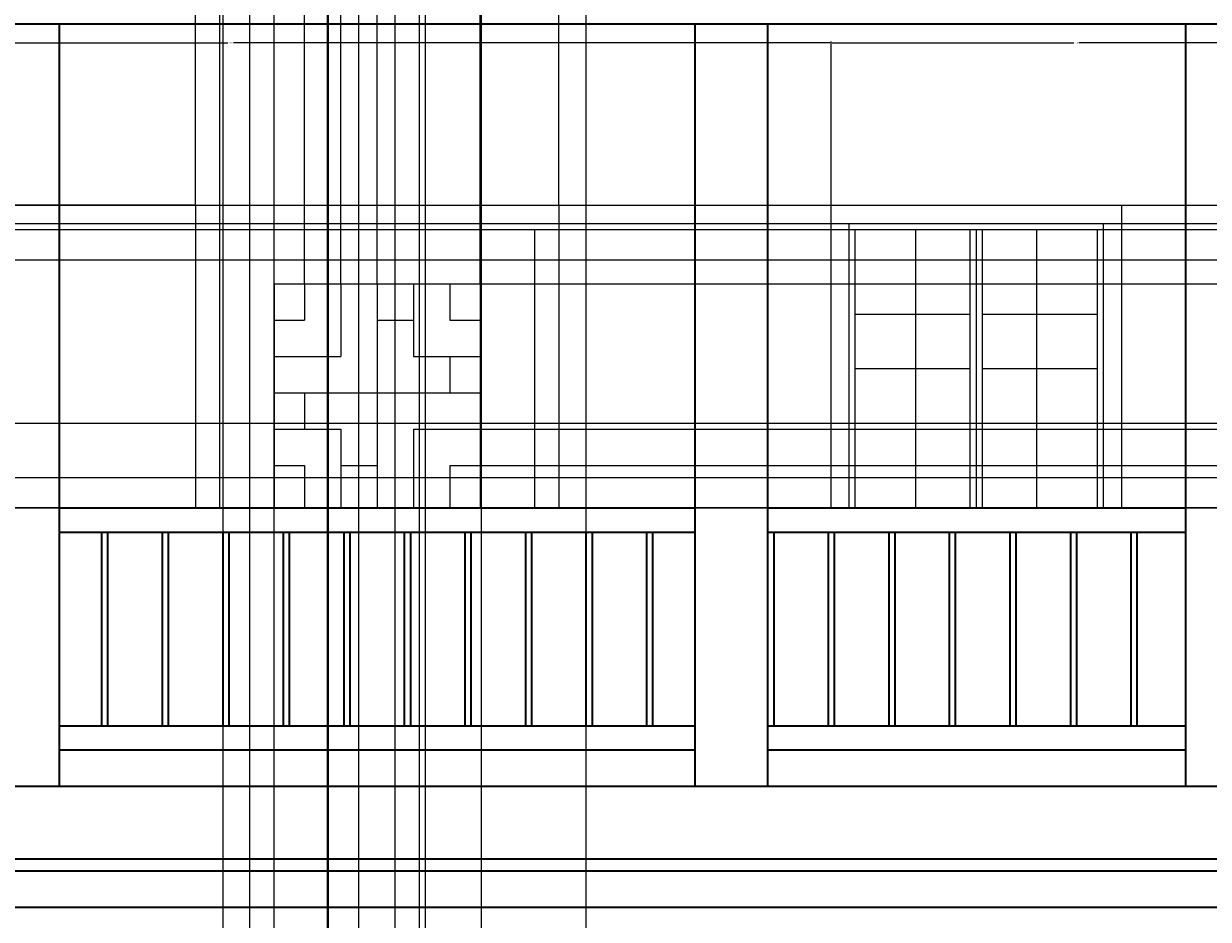
# Model space of a CAD drawing. Units: inches. Extents: x 2154 to 2740, y 571 to 1084.
# Tile 8 of 13: x 2384 to 2580, y 756 to 904. Entities that reach past the tile are written whole.
import ezdxf

# ---------------------------------------------------------------- set-up
doc = ezdxf.new("R2010")
doc.units = ezdxf.units.IN
for name, color, linetype, lineweight in [('A-ANNO-DIMS', 2, 'Continuous', 18), ('A-DOOR', 3, 'Continuous', 25), ('A-ELEV', 7, 'Continuous', 35), ('A-GLAZ', 4, 'Continuous', 25), ('A-ROOF', 1, 'Continuous', 35)]:
    doc.layers.add(name, color=color, linetype=linetype, lineweight=lineweight)
doc.styles.get("Standard").update_dxf_attribs({"font": 'arial.ttf'})
doc.dimstyles.get("Standard").update_dxf_attribs({"dimtxt": 0.18, "dimasz": 0.18, "dimexe": 0.18, "dimexo": 0.0625, "dimgap": 0.09, "dimtad": 0, "dimtih": 1, "dimtoh": 1, "dimdec": 4, "dimzin": 0, "dimdsep": 46, "dimtxsty": 'Standard', "dimcen": 0.09, "dimadec": 0, "dimazin": 0, "dimtfac": 1, "dimtdec": 4, "dimtofl": 0, "dimtmove": 0, "dimatfit": 3, "dimfxl": 1, "dimtolj": 1, "dimtzin": 0, "dimarcsym": 0})

# ---------------------------------------------------------------- blocks, each defined once
blk = doc.blocks.new('WIN-ELEV-1200')
for p, q in [((0, 50), (48, 50)), ((0, 0), (0, 50)), ((48, 0), (48, 50)), ((3, 0), (3, 47)), ((3, 47), (45, 47)), ((45, 0), (45, 47)), ((4, 46), (44, 46)), ((4, 0), (4, 46)), ((14, 0), (14, 46)), ((23, 0), (23, 46)), ((24, 0), (24, 46)), ((25, 0), (25, 46)), ((34, 0), (34, 46)), ((44, 0), (44, 46)), ((4, 41), (23, 41)), ((25, 41), (44, 41)), ((4, 32), (23, 32)), ((25, 32), (44, 32)), ((4, 23), (23, 23)), ((25, 23), (44, 23)), ((4, 14), (23, 14)), ((25, 14), (44, 14)), ((4, 5), (23, 5)), ((25, 5), (44, 5))]:
    blk.add_line(p, q)
blk = doc.blocks.new('*D9')
at = {"layer": 'A-ANNO-DIMS', "color": 0, "lineweight": -2, "transparency": 16777216}
for p, q in [((2417.21, 970.47), (2417.21, 570.5)), ((2477.21, 970.47), (2477.21, 570.5)), ((2417.39, 570.68), (2446.99, 570.68)), ((2477.03, 570.68), (2447.43, 570.68))]:
    blk.add_line(p, q, dxfattribs=at)
at = {"layer": 'A-ANNO-DIMS', "color": 0, "transparency": 16777216}
for points in [[(2417.39, 570.71), (2417.39, 570.65), (2417.21, 570.68)], [(2477.03, 570.71), (2477.03, 570.65), (2477.21, 570.68)]]:
    blk.add_solid(points, dxfattribs=at)
at = {"layer": 'Defpoints', "color": 0, "transparency": 16777216}
for p in [(2417.21, 970.53), (2477.21, 970.53), (2477.21, 570.68)]:
    blk.add_point(p, dxfattribs=at)
at = {"layer": 'A-ANNO-DIMS', "color": 0, "transparency": 16777216, "insert": (2447.21, 570.68), "char_height": 0.18, "attachment_point": 5}
blk.add_mtext('\\A1;60', dxfattribs=at)
blk = doc.blocks.new('*D10')
at = {"layer": 'A-ANNO-DIMS', "color": 0, "lineweight": -2, "transparency": 16777216}
for p, q in [((2447.14, 1057.01), (2154.18, 1057.01)), ((2154.36, 1056.83), (2154.36, 827.45)), ((2154.36, 597.71), (2154.36, 827.09)), ((2181.14, 597.53), (2154.18, 597.53))]:
    blk.add_line(p, q, dxfattribs=at)
at = {"layer": 'A-ANNO-DIMS', "color": 0, "transparency": 16777216}
for points in [[(2154.33, 1056.83), (2154.39, 1056.83), (2154.36, 1057.01)], [(2154.33, 597.71), (2154.39, 597.71), (2154.36, 597.53)]]:
    blk.add_solid(points, dxfattribs=at)
at = {"layer": 'Defpoints', "color": 0, "transparency": 16777216}
for p in [(2154.36, 1057.01), (2447.21, 1057.01), (2181.21, 597.53)]:
    blk.add_point(p, dxfattribs=at)
at = {"layer": 'A-ANNO-DIMS', "color": 0, "transparency": 16777216, "insert": (2154.36, 827.27), "char_height": 0.18, "attachment_point": 5}
blk.add_mtext('\\A1;459.5', dxfattribs=at)
blk = doc.blocks.new('*D30')
at = {"layer": 'A-ANNO-DIMS', "color": 0, "lineweight": -2, "transparency": 16777216}
for p, q in [((2657.14, 823.53), (2154.18, 823.53)), ((2154.36, 823.35), (2154.36, 800.71)), ((2154.36, 777.71), (2154.36, 800.35)), ((2657.14, 777.53), (2154.18, 777.53))]:
    blk.add_line(p, q, dxfattribs=at)
at = {"layer": 'A-ANNO-DIMS', "color": 0, "transparency": 16777216}
for points in [[(2154.33, 823.35), (2154.39, 823.35), (2154.36, 823.53)], [(2154.33, 777.71), (2154.39, 777.71), (2154.36, 777.53)]]:
    blk.add_solid(points, dxfattribs=at)
at = {"layer": 'Defpoints', "color": 0, "transparency": 16777216}
for p in [(2154.36, 823.53), (2657.21, 823.53), (2657.21, 777.53)]:
    blk.add_point(p, dxfattribs=at)
at = {"layer": 'A-ANNO-DIMS', "color": 0, "transparency": 16777216, "insert": (2154.36, 800.53), "char_height": 0.18, "attachment_point": 5}
blk.add_mtext('\\A1;46', dxfattribs=at)
blk = doc.blocks.new('*D32')
at = {"layer": 'A-ANNO-DIMS', "color": 0, "lineweight": -2, "transparency": 16777216}
for p, q in [((2412.71, 873.59), (2412.71, 1084.04)), ((2472.71, 873.59), (2472.71, 1084.04)), ((2412.89, 1083.86), (2442.49, 1083.86)), ((2472.53, 1083.86), (2442.93, 1083.86))]:
    blk.add_line(p, q, dxfattribs=at)
at = {"layer": 'A-ANNO-DIMS', "color": 0, "transparency": 16777216}
for points in [[(2412.89, 1083.89), (2412.89, 1083.83), (2412.71, 1083.86)], [(2472.53, 1083.89), (2472.53, 1083.83), (2472.71, 1083.86)]]:
    blk.add_solid(points, dxfattribs=at)
at = {"layer": 'Defpoints', "color": 0, "transparency": 16777216}
for p in [(2472.71, 1083.86), (2412.71, 873.53), (2472.71, 873.53)]:
    blk.add_point(p, dxfattribs=at)
at = {"layer": 'A-ANNO-DIMS', "color": 0, "transparency": 16777216, "insert": (2442.71, 1083.86), "char_height": 0.18, "attachment_point": 5}
blk.add_mtext('\\A1;60', dxfattribs=at)
blk = doc.blocks.new('*D33')
at = {"layer": 'A-ANNO-DIMS', "color": 0, "lineweight": -2, "transparency": 16777216}
for p, q in [((2412.64, 873.53), (2154.18, 873.53)), ((2154.36, 873.35), (2154.36, 848.71)), ((2154.36, 823.71), (2154.36, 848.35)), ((2412.64, 823.53), (2154.18, 823.53))]:
    blk.add_line(p, q, dxfattribs=at)
at = {"layer": 'A-ANNO-DIMS', "color": 0, "transparency": 16777216}
for points in [[(2154.33, 873.35), (2154.39, 873.35), (2154.36, 873.53)], [(2154.33, 823.71), (2154.39, 823.71), (2154.36, 823.53)]]:
    blk.add_solid(points, dxfattribs=at)
at = {"layer": 'Defpoints', "color": 0, "transparency": 16777216}
for p in [(2154.36, 873.53), (2412.71, 873.53), (2412.71, 823.53)]:
    blk.add_point(p, dxfattribs=at)
at = {"layer": 'A-ANNO-DIMS', "color": 0, "transparency": 16777216, "insert": (2154.36, 848.53), "char_height": 0.18, "attachment_point": 5}
blk.add_mtext('\\A1;50', dxfattribs=at)
blk = doc.blocks.new('*D39')
at = {"layer": 'A-ANNO-DIMS', "color": 0, "lineweight": -2, "transparency": 16777216}
for p, q in [((2183.21, 979.47), (2183.21, 570.5)), ((2417.21, 970.47), (2417.21, 570.5)), ((2183.39, 570.68), (2299.92, 570.68)), ((2417.03, 570.68), (2300.5, 570.68))]:
    blk.add_line(p, q, dxfattribs=at)
at = {"layer": 'A-ANNO-DIMS', "color": 0, "transparency": 16777216}
for points in [[(2183.39, 570.71), (2183.39, 570.65), (2183.21, 570.68)], [(2417.03, 570.71), (2417.03, 570.65), (2417.21, 570.68)]]:
    blk.add_solid(points, dxfattribs=at)
at = {"layer": 'Defpoints', "color": 0, "transparency": 16777216}
for p in [(2183.21, 979.53), (2417.21, 970.53), (2417.21, 570.68)]:
    blk.add_point(p, dxfattribs=at)
at = {"layer": 'A-ANNO-DIMS', "color": 0, "transparency": 16777216, "insert": (2300.21, 570.68), "char_height": 0.18, "attachment_point": 5}
blk.add_mtext('\\A1;234', dxfattribs=at)
blk = doc.blocks.new('*D41')
at = {"layer": 'A-ANNO-DIMS', "color": 0, "lineweight": -2, "transparency": 16777216}
for p, q in [((2319.35, 873.59), (2319.35, 900.56)), ((2319.53, 900.38), (2418.06, 900.38)), ((2517.5, 900.38), (2418.97, 900.38)), ((2517.68, 873.59), (2517.68, 900.56))]:
    blk.add_line(p, q, dxfattribs=at)
at = {"layer": 'A-ANNO-DIMS', "color": 0, "transparency": 16777216}
for points in [[(2319.53, 900.41), (2319.53, 900.35), (2319.35, 900.38)], [(2517.5, 900.41), (2517.5, 900.35), (2517.68, 900.38)]]:
    blk.add_solid(points, dxfattribs=at)
at = {"layer": 'Defpoints', "color": 0, "transparency": 16777216}
for p in [(2517.68, 900.38), (2319.35, 873.53), (2517.68, 873.53)]:
    blk.add_point(p, dxfattribs=at)
at = {"layer": 'A-ANNO-DIMS', "color": 0, "transparency": 16777216, "insert": (2418.51, 900.38), "char_height": 0.18, "attachment_point": 5}
blk.add_mtext('\\A1;198.33', dxfattribs=at)
blk = doc.blocks.new('*D42')
at = {"layer": 'A-ANNO-DIMS', "color": 0, "lineweight": -2, "transparency": 16777216}
for p, q in [((2517.68, 873.59), (2517.68, 900.56)), ((2517.86, 900.38), (2557.8, 900.38)), ((2598.53, 900.38), (2558.59, 900.38)), ((2598.71, 873.59), (2598.71, 900.56))]:
    blk.add_line(p, q, dxfattribs=at)
at = {"layer": 'A-ANNO-DIMS', "color": 0, "transparency": 16777216}
for points in [[(2517.86, 900.41), (2517.86, 900.35), (2517.68, 900.38)], [(2598.53, 900.41), (2598.53, 900.35), (2598.71, 900.38)]]:
    blk.add_solid(points, dxfattribs=at)
at = {"layer": 'Defpoints', "color": 0, "transparency": 16777216}
for p in [(2598.71, 900.38), (2517.68, 873.53), (2598.71, 873.53)]:
    blk.add_point(p, dxfattribs=at)
at = {"layer": 'A-ANNO-DIMS', "color": 0, "transparency": 16777216, "insert": (2558.19, 900.38), "char_height": 0.18, "attachment_point": 5}
blk.add_mtext('\\A1;81.03', dxfattribs=at)
blk = doc.blocks.new('*D75')
at = {"layer": 'A-ANNO-DIMS', "color": 0, "lineweight": -2, "transparency": 16777216}
for p, q in [((2434.46, 990.57), (2434.46, 570.5)), ((2417.21, 981.47), (2417.21, 570.5)), ((2417.39, 570.68), (2425.45, 570.68)), ((2434.28, 570.68), (2426.22, 570.68))]:
    blk.add_line(p, q, dxfattribs=at)
at = {"layer": 'A-ANNO-DIMS', "color": 0, "transparency": 16777216}
for points in [[(2417.39, 570.71), (2417.39, 570.65), (2417.21, 570.68)], [(2434.28, 570.71), (2434.28, 570.65), (2434.46, 570.68)]]:
    blk.add_solid(points, dxfattribs=at)
at = {"layer": 'Defpoints', "color": 0, "transparency": 16777216}
for p in [(2434.46, 990.64), (2417.21, 981.53), (2434.46, 570.68)]:
    blk.add_point(p, dxfattribs=at)
at = {"layer": 'A-ANNO-DIMS', "color": 0, "transparency": 16777216, "insert": (2425.83, 570.68), "char_height": 0.18, "attachment_point": 5}
blk.add_mtext('\\A1;17.25', dxfattribs=at)
blk = doc.blocks.new('*D76')
at = {"layer": 'A-ANNO-DIMS', "color": 0, "lineweight": -2, "transparency": 16777216}
for p, q in [((2434.46, 990.57), (2434.46, 570.5)), ((2459.89, 990.57), (2459.89, 570.5)), ((2434.64, 570.68), (2446.71, 570.68)), ((2459.71, 570.68), (2447.64, 570.68))]:
    blk.add_line(p, q, dxfattribs=at)
at = {"layer": 'A-ANNO-DIMS', "color": 0, "transparency": 16777216}
for points in [[(2434.64, 570.71), (2434.64, 570.65), (2434.46, 570.68)], [(2459.71, 570.71), (2459.71, 570.65), (2459.89, 570.68)]]:
    blk.add_solid(points, dxfattribs=at)
at = {"layer": 'Defpoints', "color": 0, "transparency": 16777216}
for p in [(2434.46, 990.64), (2459.89, 990.64), (2459.89, 570.68)]:
    blk.add_point(p, dxfattribs=at)
at = {"layer": 'A-ANNO-DIMS', "color": 0, "transparency": 16777216, "insert": (2447.17, 570.68), "char_height": 0.18, "attachment_point": 5}
blk.add_mtext('\\A1;25.433', dxfattribs=at)
blk = doc.blocks.new('*D87')
at = {"layer": 'A-ANNO-DIMS', "color": 0, "lineweight": -2, "transparency": 16777216}
for p, q in [((2421.71, 725.29), (2421.71, 1084.04)), ((2425.71, 721.29), (2425.71, 1084.04)), ((2421.89, 1083.86), (2423.55, 1083.86)), ((2425.53, 1083.86), (2423.86, 1083.86))]:
    blk.add_line(p, q, dxfattribs=at)
at = {"layer": 'A-ANNO-DIMS', "color": 0, "transparency": 16777216}
for points in [[(2421.89, 1083.89), (2421.89, 1083.83), (2421.71, 1083.86)], [(2425.53, 1083.89), (2425.53, 1083.83), (2425.71, 1083.86)]]:
    blk.add_solid(points, dxfattribs=at)
at = {"layer": 'Defpoints', "color": 0, "transparency": 16777216}
for p in [(2425.71, 1083.86), (2421.71, 725.23), (2425.71, 721.23)]:
    blk.add_point(p, dxfattribs=at)
at = {"layer": 'A-ANNO-DIMS', "color": 0, "transparency": 16777216, "insert": (2423.71, 1083.86), "char_height": 0.18, "attachment_point": 5}
blk.add_mtext('\\A1;4', dxfattribs=at)
blk = doc.blocks.new('*D90')
at = {"layer": 'A-ANNO-DIMS', "color": 0, "lineweight": -2, "transparency": 16777216}
for p, q in [((2434.71, 712.29), (2434.71, 1084.04)), ((2450.71, 712.29), (2450.71, 1084.04)), ((2434.89, 1083.86), (2442.5, 1083.86)), ((2450.53, 1083.86), (2442.92, 1083.86))]:
    blk.add_line(p, q, dxfattribs=at)
at = {"layer": 'A-ANNO-DIMS', "color": 0, "transparency": 16777216}
for points in [[(2434.89, 1083.89), (2434.89, 1083.83), (2434.71, 1083.86)], [(2450.53, 1083.89), (2450.53, 1083.83), (2450.71, 1083.86)]]:
    blk.add_solid(points, dxfattribs=at)
at = {"layer": 'Defpoints', "color": 0, "transparency": 16777216}
for p in [(2450.71, 1083.86), (2434.71, 712.23), (2450.71, 712.23)]:
    blk.add_point(p, dxfattribs=at)
at = {"layer": 'A-ANNO-DIMS', "color": 0, "transparency": 16777216, "insert": (2442.71, 1083.86), "char_height": 0.18, "attachment_point": 5}
blk.add_mtext('\\A1;16', dxfattribs=at)
blk = doc.blocks.new('*D93')
at = {"layer": 'A-ANNO-DIMS', "color": 0, "lineweight": -2, "transparency": 16777216}
for p, q in [((2439.71, 703.29), (2439.71, 1084.04)), ((2445.71, 703.29), (2445.71, 1084.04)), ((2439.89, 1083.86), (2442.56, 1083.86)), ((2445.53, 1083.86), (2442.86, 1083.86))]:
    blk.add_line(p, q, dxfattribs=at)
at = {"layer": 'A-ANNO-DIMS', "color": 0, "transparency": 16777216}
for points in [[(2439.89, 1083.89), (2439.89, 1083.83), (2439.71, 1083.86)], [(2445.53, 1083.89), (2445.53, 1083.83), (2445.71, 1083.86)]]:
    blk.add_solid(points, dxfattribs=at)
at = {"layer": 'Defpoints', "color": 0, "transparency": 16777216}
for p in [(2445.71, 1083.86), (2439.71, 703.23), (2445.71, 703.23)]:
    blk.add_point(p, dxfattribs=at)
at = {"layer": 'A-ANNO-DIMS', "color": 0, "transparency": 16777216, "insert": (2442.71, 1083.86), "char_height": 0.18, "attachment_point": 5}
blk.add_mtext('\\A1;6', dxfattribs=at)
blk = doc.blocks.new('*D94')
at = {"layer": 'A-ANNO-DIMS', "color": 0, "lineweight": -2, "transparency": 16777216}
for p, q in [((2445.71, 703.29), (2445.71, 1084.04)), ((2449.71, 703.29), (2449.71, 1084.04)), ((2445.89, 1083.86), (2447.55, 1083.86)), ((2449.53, 1083.86), (2447.86, 1083.86))]:
    blk.add_line(p, q, dxfattribs=at)
at = {"layer": 'A-ANNO-DIMS', "color": 0, "transparency": 16777216}
for points in [[(2445.89, 1083.89), (2445.89, 1083.83), (2445.71, 1083.86)], [(2449.53, 1083.89), (2449.53, 1083.83), (2449.71, 1083.86)]]:
    blk.add_solid(points, dxfattribs=at)
at = {"layer": 'Defpoints', "color": 0, "transparency": 16777216}
for p in [(2449.71, 1083.86), (2445.71, 703.23), (2449.71, 703.23)]:
    blk.add_point(p, dxfattribs=at)
at = {"layer": 'A-ANNO-DIMS', "color": 0, "transparency": 16777216, "insert": (2447.71, 1083.86), "char_height": 0.18, "attachment_point": 5}
blk.add_mtext('\\A1;4', dxfattribs=at)
blk = doc.blocks.new('*D99')
at = {"layer": 'A-ANNO-DIMS', "color": 0, "lineweight": -2, "transparency": 16777216}
for p, q in [((2412.71, 873.59), (2412.71, 1084.04)), ((2416.71, 869.59), (2416.71, 1084.04)), ((2412.89, 1083.86), (2414.55, 1083.86)), ((2416.53, 1083.86), (2414.86, 1083.86))]:
    blk.add_line(p, q, dxfattribs=at)
at = {"layer": 'A-ANNO-DIMS', "color": 0, "transparency": 16777216}
for points in [[(2412.89, 1083.89), (2412.89, 1083.83), (2412.71, 1083.86)], [(2416.53, 1083.89), (2416.53, 1083.83), (2416.71, 1083.86)]]:
    blk.add_solid(points, dxfattribs=at)
at = {"layer": 'Defpoints', "color": 0, "transparency": 16777216}
for p in [(2416.71, 1083.86), (2412.71, 873.53), (2416.71, 869.53)]:
    blk.add_point(p, dxfattribs=at)
at = {"layer": 'A-ANNO-DIMS', "color": 0, "transparency": 16777216, "insert": (2414.71, 1083.86), "char_height": 0.18, "attachment_point": 5}
blk.add_mtext('\\A1;4', dxfattribs=at)
blk = doc.blocks.new('*D100')
at = {"layer": 'A-ANNO-DIMS', "color": 0, "lineweight": -2, "transparency": 16777216}
for p, q in [((2472.769199, 873.532069), (2740.236699, 873.532069)), ((2740.056699, 873.352069), (2740.056699, 871.712069)), ((2740.056699, 869.712069), (2740.056699, 871.352069)), ((2468.769199, 869.532069), (2740.236699, 869.532069))]:
    blk.add_line(p, q, dxfattribs=at)
at = {"layer": 'A-ANNO-DIMS', "color": 0, "transparency": 16777216}
for points in [[(2740.026699, 873.352069), (2740.086699, 873.352069), (2740.056699, 873.532069)], [(2740.026699, 869.712069), (2740.086699, 869.712069), (2740.056699, 869.532069)]]:
    blk.add_solid(points, dxfattribs=at)
at = {"layer": 'Defpoints', "color": 0, "transparency": 16777216}
for p in [(2472.706699, 873.532069), (2468.706699, 869.532069), (2740.056699, 869.532069)]:
    blk.add_point(p, dxfattribs=at)
at = {"layer": 'A-ANNO-DIMS', "color": 0, "transparency": 16777216, "insert": (2740.056699, 871.532069), "char_height": 0.18, "attachment_point": 5}
blk.add_mtext('\\A1;4', dxfattribs=at)
blk = doc.blocks.new('*D101')
at = {"layer": 'A-ANNO-DIMS', "color": 0, "lineweight": -2, "transparency": 16777216}
for p, q in [((2416.71, 869.59), (2416.71, 1084.04)), ((2425.71, 860.59), (2425.71, 1084.04)), ((2416.89, 1083.86), (2421.06, 1083.86)), ((2425.53, 1083.86), (2421.36, 1083.86))]:
    blk.add_line(p, q, dxfattribs=at)
at = {"layer": 'A-ANNO-DIMS', "color": 0, "transparency": 16777216}
for points in [[(2416.89, 1083.89), (2416.89, 1083.83), (2416.71, 1083.86)], [(2425.53, 1083.89), (2425.53, 1083.83), (2425.71, 1083.86)]]:
    blk.add_solid(points, dxfattribs=at)
at = {"layer": 'Defpoints', "color": 0, "transparency": 16777216}
for p in [(2425.71, 1083.86), (2416.71, 869.53), (2425.71, 860.53)]:
    blk.add_point(p, dxfattribs=at)
at = {"layer": 'A-ANNO-DIMS', "color": 0, "transparency": 16777216, "insert": (2421.21, 1083.86), "char_height": 0.18, "attachment_point": 5}
blk.add_mtext('\\A1;9', dxfattribs=at)
blk = doc.blocks.new('*D102')
at = {"layer": 'A-ANNO-DIMS', "color": 0, "lineweight": -2, "transparency": 16777216}
for p, q in [((2425.71, 860.59), (2425.71, 1084.04)), ((2430.71, 860.59), (2430.71, 1084.04)), ((2425.89, 1083.86), (2428.06, 1083.86)), ((2430.53, 1083.86), (2428.36, 1083.86))]:
    blk.add_line(p, q, dxfattribs=at)
at = {"layer": 'A-ANNO-DIMS', "color": 0, "transparency": 16777216}
for points in [[(2425.89, 1083.89), (2425.89, 1083.83), (2425.71, 1083.86)], [(2430.53, 1083.89), (2430.53, 1083.83), (2430.71, 1083.86)]]:
    blk.add_solid(points, dxfattribs=at)
at = {"layer": 'Defpoints', "color": 0, "transparency": 16777216}
for p in [(2430.71, 1083.86), (2425.71, 860.53), (2430.71, 860.53)]:
    blk.add_point(p, dxfattribs=at)
at = {"layer": 'A-ANNO-DIMS', "color": 0, "transparency": 16777216, "insert": (2428.21, 1083.86), "char_height": 0.18, "attachment_point": 5}
blk.add_mtext('\\A1;5', dxfattribs=at)
blk = doc.blocks.new('*D103')
at = {"layer": 'A-ANNO-DIMS', "color": 0, "lineweight": -2, "transparency": 16777216}
for p, q in [((2430.71, 860.59), (2430.71, 1084.04)), ((2436.71, 860.59), (2436.71, 1084.04)), ((2430.89, 1083.86), (2433.56, 1083.86)), ((2436.53, 1083.86), (2433.86, 1083.86))]:
    blk.add_line(p, q, dxfattribs=at)
at = {"layer": 'A-ANNO-DIMS', "color": 0, "transparency": 16777216}
for points in [[(2430.89, 1083.89), (2430.89, 1083.83), (2430.71, 1083.86)], [(2436.53, 1083.89), (2436.53, 1083.83), (2436.71, 1083.86)]]:
    blk.add_solid(points, dxfattribs=at)
at = {"layer": 'Defpoints', "color": 0, "transparency": 16777216}
for p in [(2436.71, 1083.86), (2430.71, 860.53), (2436.71, 860.53)]:
    blk.add_point(p, dxfattribs=at)
at = {"layer": 'A-ANNO-DIMS', "color": 0, "transparency": 16777216, "insert": (2433.71, 1083.86), "char_height": 0.18, "attachment_point": 5}
blk.add_mtext('\\A1;6', dxfattribs=at)
blk = doc.blocks.new('*D104')
at = {"layer": 'A-ANNO-DIMS', "color": 0, "lineweight": -2, "transparency": 16777216}
for p, q in [((2436.71, 860.59), (2436.71, 1084.04)), ((2442.71, 860.59), (2442.71, 1084.04)), ((2436.89, 1083.86), (2439.56, 1083.86)), ((2442.53, 1083.86), (2439.86, 1083.86))]:
    blk.add_line(p, q, dxfattribs=at)
at = {"layer": 'A-ANNO-DIMS', "color": 0, "transparency": 16777216}
for points in [[(2436.89, 1083.89), (2436.89, 1083.83), (2436.71, 1083.86)], [(2442.53, 1083.89), (2442.53, 1083.83), (2442.71, 1083.86)]]:
    blk.add_solid(points, dxfattribs=at)
at = {"layer": 'Defpoints', "color": 0, "transparency": 16777216}
for p in [(2442.71, 1083.86), (2436.71, 860.53), (2442.71, 860.53)]:
    blk.add_point(p, dxfattribs=at)
at = {"layer": 'A-ANNO-DIMS', "color": 0, "transparency": 16777216, "insert": (2439.71, 1083.86), "char_height": 0.18, "attachment_point": 5}
blk.add_mtext('\\A1;6', dxfattribs=at)
blk = doc.blocks.new('*D105')
at = {"layer": 'A-ANNO-DIMS', "color": 0, "lineweight": -2, "transparency": 16777216}
for p, q in [((2442.71, 860.59), (2442.71, 1084.04)), ((2459.71, 860.59), (2459.71, 1084.04)), ((2442.89, 1083.86), (2451, 1083.86)), ((2459.53, 1083.86), (2451.42, 1083.86))]:
    blk.add_line(p, q, dxfattribs=at)
at = {"layer": 'A-ANNO-DIMS', "color": 0, "transparency": 16777216}
for points in [[(2442.89, 1083.89), (2442.89, 1083.83), (2442.71, 1083.86)], [(2459.53, 1083.89), (2459.53, 1083.83), (2459.71, 1083.86)]]:
    blk.add_solid(points, dxfattribs=at)
at = {"layer": 'Defpoints', "color": 0, "transparency": 16777216}
for p in [(2459.71, 1083.86), (2442.71, 860.53), (2459.71, 860.53)]:
    blk.add_point(p, dxfattribs=at)
at = {"layer": 'A-ANNO-DIMS', "color": 0, "transparency": 16777216, "insert": (2451.21, 1083.86), "char_height": 0.18, "attachment_point": 5}
blk.add_mtext('\\A1;17', dxfattribs=at)
blk = doc.blocks.new('*D106')
at = {"layer": 'A-ANNO-DIMS', "color": 0, "lineweight": -2, "transparency": 16777216}
for p, q in [((2459.769199, 830.532069), (2740.236699, 830.532069)), ((2740.056699, 830.352069), (2740.056699, 827.212069)), ((2740.056699, 823.712069), (2740.056699, 826.852069)), ((2459.769199, 823.532069), (2740.236699, 823.532069))]:
    blk.add_line(p, q, dxfattribs=at)
at = {"layer": 'A-ANNO-DIMS', "color": 0, "transparency": 16777216}
for points in [[(2740.026699, 830.352069), (2740.086699, 830.352069), (2740.056699, 830.532069)], [(2740.026699, 823.712069), (2740.086699, 823.712069), (2740.056699, 823.532069)]]:
    blk.add_solid(points, dxfattribs=at)
at = {"layer": 'Defpoints', "color": 0, "transparency": 16777216}
for p in [(2459.706699, 830.532069), (2740.056699, 830.532069), (2459.706699, 823.532069)]:
    blk.add_point(p, dxfattribs=at)
at = {"layer": 'A-ANNO-DIMS', "color": 0, "transparency": 16777216, "insert": (2740.056699, 827.032069), "char_height": 0.18, "attachment_point": 5}
blk.add_mtext('\\A1;7', dxfattribs=at)
blk = doc.blocks.new('*D107')
at = {"layer": 'A-ANNO-DIMS', "color": 0, "lineweight": -2, "transparency": 16777216}
for p, q in [((2459.77, 836.53), (2740.24, 836.53)), ((2740.06, 836.35), (2740.06, 833.71)), ((2740.06, 830.71), (2740.06, 833.35)), ((2459.77, 830.53), (2740.24, 830.53))]:
    blk.add_line(p, q, dxfattribs=at)
at = {"layer": 'A-ANNO-DIMS', "color": 0, "transparency": 16777216}
for points in [[(2740.03, 836.35), (2740.09, 836.35), (2740.06, 836.53)], [(2740.03, 830.71), (2740.09, 830.71), (2740.06, 830.53)]]:
    blk.add_solid(points, dxfattribs=at)
at = {"layer": 'Defpoints', "color": 0, "transparency": 16777216}
for p in [(2459.71, 836.53), (2740.06, 836.53), (2459.71, 830.53)]:
    blk.add_point(p, dxfattribs=at)
at = {"layer": 'A-ANNO-DIMS', "color": 0, "transparency": 16777216, "insert": (2740.06, 833.53), "char_height": 0.18, "attachment_point": 5}
blk.add_mtext('\\A1;6', dxfattribs=at)
blk = doc.blocks.new('*D108')
at = {"layer": 'A-ANNO-DIMS', "color": 0, "lineweight": -2, "transparency": 16777216}
for p, q in [((2459.77, 860.53), (2740.24, 860.53)), ((2740.06, 860.35), (2740.06, 848.71)), ((2740.06, 836.71), (2740.06, 848.35)), ((2459.77, 836.53), (2740.24, 836.53))]:
    blk.add_line(p, q, dxfattribs=at)
at = {"layer": 'A-ANNO-DIMS', "color": 0, "transparency": 16777216}
for points in [[(2740.03, 860.35), (2740.09, 860.35), (2740.06, 860.53)], [(2740.03, 836.71), (2740.09, 836.71), (2740.06, 836.53)]]:
    blk.add_solid(points, dxfattribs=at)
at = {"layer": 'Defpoints', "color": 0, "transparency": 16777216}
for p in [(2459.71, 860.53), (2740.06, 860.53), (2459.71, 836.53)]:
    blk.add_point(p, dxfattribs=at)
at = {"layer": 'A-ANNO-DIMS', "color": 0, "transparency": 16777216, "insert": (2740.06, 848.53), "char_height": 0.18, "attachment_point": 5}
blk.add_mtext('\\A1;24', dxfattribs=at)
blk = doc.blocks.new('*D109')
at = {"layer": 'A-ANNO-DIMS', "color": 0, "lineweight": -2, "transparency": 16777216}
for p, q in [((2468.77, 869.53), (2740.24, 869.53)), ((2740.06, 869.35), (2740.06, 865.21)), ((2740.06, 860.71), (2740.06, 864.85)), ((2459.77, 860.53), (2740.24, 860.53))]:
    blk.add_line(p, q, dxfattribs=at)
at = {"layer": 'A-ANNO-DIMS', "color": 0, "transparency": 16777216}
for points in [[(2740.03, 869.35), (2740.09, 869.35), (2740.06, 869.53)], [(2740.03, 860.71), (2740.09, 860.71), (2740.06, 860.53)]]:
    blk.add_solid(points, dxfattribs=at)
at = {"layer": 'Defpoints', "color": 0, "transparency": 16777216}
for p in [(2468.71, 869.53), (2740.06, 869.53), (2459.71, 860.53)]:
    blk.add_point(p, dxfattribs=at)
at = {"layer": 'A-ANNO-DIMS', "color": 0, "transparency": 16777216, "insert": (2740.06, 865.03), "char_height": 0.18, "attachment_point": 5}
blk.add_mtext('\\A1;9', dxfattribs=at)
blk = doc.blocks.new('*D112')
at = {"layer": 'A-ANNO-DIMS', "color": 0, "lineweight": -2, "transparency": 16777216}
for p, q in [((2291.32, 873.53), (2740.24, 873.53)), ((2740.06, 873.35), (2740.06, 872.21)), ((2740.06, 870.71), (2740.06, 871.85)), ((2288.32, 870.53), (2740.24, 870.53))]:
    blk.add_line(p, q, dxfattribs=at)
at = {"layer": 'A-ANNO-DIMS', "color": 0, "transparency": 16777216}
for points in [[(2740.03, 873.35), (2740.09, 873.35), (2740.06, 873.53)], [(2740.03, 870.71), (2740.09, 870.71), (2740.06, 870.53)]]:
    blk.add_solid(points, dxfattribs=at)
at = {"layer": 'Defpoints', "color": 0, "transparency": 16777216}
for p in [(2291.26, 873.53), (2740.06, 873.53), (2288.26, 870.53)]:
    blk.add_point(p, dxfattribs=at)
at = {"layer": 'A-ANNO-DIMS', "color": 0, "transparency": 16777216, "insert": (2740.06, 872.03), "char_height": 0.18, "attachment_point": 5}
blk.add_mtext('\\A1;3', dxfattribs=at)
blk = doc.blocks.new('*D119')
at = {"layer": 'A-ANNO-DIMS', "color": 0, "lineweight": -2, "transparency": 16777216}
for p, q in [((2287.32, 828.53), (2740.24, 828.53)), ((2740.06, 828.35), (2740.06, 826.21)), ((2740.06, 823.71), (2740.06, 825.85)), ((2287.32, 823.53), (2740.24, 823.53))]:
    blk.add_line(p, q, dxfattribs=at)
at = {"layer": 'A-ANNO-DIMS', "color": 0, "transparency": 16777216}
for points in [[(2740.03, 828.35), (2740.09, 828.35), (2740.06, 828.53)], [(2740.03, 823.71), (2740.09, 823.71), (2740.06, 823.53)]]:
    blk.add_solid(points, dxfattribs=at)
at = {"layer": 'Defpoints', "color": 0, "transparency": 16777216}
for p in [(2287.26, 828.53), (2740.06, 828.53), (2287.26, 823.53)]:
    blk.add_point(p, dxfattribs=at)
at = {"layer": 'A-ANNO-DIMS', "color": 0, "transparency": 16777216, "insert": (2740.06, 826.03), "char_height": 0.18, "attachment_point": 5}
blk.add_mtext('\\A1;5', dxfattribs=at)
blk = doc.blocks.new('*D120')
at = {"layer": 'A-ANNO-DIMS', "color": 0, "lineweight": -2, "transparency": 16777216}
for p, q in [((2287.32, 837.53), (2740.24, 837.53)), ((2740.06, 837.35), (2740.06, 833.21)), ((2740.06, 828.71), (2740.06, 832.85)), ((2287.32, 828.53), (2740.24, 828.53))]:
    blk.add_line(p, q, dxfattribs=at)
at = {"layer": 'A-ANNO-DIMS', "color": 0, "transparency": 16777216}
for points in [[(2740.03, 837.35), (2740.09, 837.35), (2740.06, 837.53)], [(2740.03, 828.71), (2740.09, 828.71), (2740.06, 828.53)]]:
    blk.add_solid(points, dxfattribs=at)
at = {"layer": 'Defpoints', "color": 0, "transparency": 16777216}
for p in [(2287.26, 837.53), (2740.06, 837.53), (2287.26, 828.53)]:
    blk.add_point(p, dxfattribs=at)
at = {"layer": 'A-ANNO-DIMS', "color": 0, "transparency": 16777216, "insert": (2740.06, 833.03), "char_height": 0.18, "attachment_point": 5}
blk.add_mtext('\\A1;9', dxfattribs=at)
blk = doc.blocks.new('*D121')
at = {"layer": 'A-ANNO-DIMS', "color": 0, "lineweight": -2, "transparency": 16777216}
for p, q in [((2287.32, 869.53), (2740.24, 869.53)), ((2740.06, 869.35), (2740.06, 867.21)), ((2740.06, 864.71), (2740.06, 866.85)), ((2287.32, 864.53), (2740.24, 864.53))]:
    blk.add_line(p, q, dxfattribs=at)
at = {"layer": 'A-ANNO-DIMS', "color": 0, "transparency": 16777216}
for points in [[(2740.03, 869.35), (2740.09, 869.35), (2740.06, 869.53)], [(2740.03, 864.71), (2740.09, 864.71), (2740.06, 864.53)]]:
    blk.add_solid(points, dxfattribs=at)
at = {"layer": 'Defpoints', "color": 0, "transparency": 16777216}
for p in [(2287.26, 869.53), (2740.06, 869.53), (2287.26, 864.53)]:
    blk.add_point(p, dxfattribs=at)
at = {"layer": 'A-ANNO-DIMS', "color": 0, "transparency": 16777216, "insert": (2740.06, 867.03), "char_height": 0.18, "attachment_point": 5}
blk.add_mtext('\\A1;5', dxfattribs=at)

msp = doc.modelspace()

# ---------------------------------------------------------------- linework, layer by layer
at = {"layer": 'A-DOOR'}
for p, q in [((2412.7067, 873.5321), (2472.7067, 873.5321)), ((2412.7067, 873.5321), (2412.7067, 823.5321)), ((2472.7067, 873.5321), (2472.7067, 823.5321)), ((2416.7067, 869.5321), (2468.7067, 869.5321)), ((2416.7067, 869.5321), (2416.7067, 823.5321)), ((2468.7067, 869.5321), (2468.7067, 823.5321)), ((2425.7067, 860.5321), (2425.7067, 823.5321)), ((2425.7067, 860.5321), (2459.7067, 860.5321)), ((2430.7067, 860.5321), (2430.7067, 854.5321)), ((2436.7067, 860.5321), (2436.7067, 848.5321)), ((2442.7067, 860.5321), (2442.7067, 823.5321)), ((2448.7067, 860.5321), (2448.7067, 848.5321)), ((2454.7067, 860.5321), (2454.7067, 854.5321)), ((2459.7067, 860.5321), (2459.7067, 823.5321)), ((2425.7067, 854.5321), (2430.7067, 854.5321)), ((2442.7067, 854.5321), (2448.7067, 854.5321)), ((2454.7067, 854.5321), (2459.7067, 854.5321)), ((2425.7067, 848.5321), (2436.7067, 848.5321)), ((2448.7067, 848.5321), (2459.7067, 848.5321)), ((2454.7067, 848.5321), (2454.7067, 842.5321)), ((2425.7067, 842.5321), (2459.7067, 842.5321)), ((2430.7067, 842.5321), (2430.7067, 836.5321)), ((2425.7067, 836.5321), (2436.7067, 836.5321)), ((2436.7067, 836.5321), (2436.7067, 823.5321)), ((2448.7067, 836.5321), (2459.7067, 836.5321)), ((2448.7067, 836.5321), (2448.7067, 823.5321)), ((2425.7067, 830.5321), (2430.7067, 830.5321)), ((2430.7067, 830.5321), (2430.7067, 823.5321)), ((2436.7067, 830.5321), (2442.7067, 830.5321)), ((2454.7067, 830.5321), (2454.7067, 823.5321)), ((2454.7067, 830.5321), (2459.7067, 830.5321))]:
    msp.add_line(p, q, dxfattribs=at)
at = {"layer": 'A-ELEV'}
for p, q in [((2390.2067, 903.5321), (2390.2067, 777.5321)), ((2495.2067, 903.5321), (2495.2067, 777.5321)), ((2507.2067, 903.5321), (2507.2067, 777.5321)), ((2576.2067, 903.5321), (2576.2067, 777.5321)), ((2390.2067, 823.5321), (2495.2067, 823.5321)), ((2507.2067, 823.5321), (2576.2067, 823.5321)), ((2390.2067, 819.5321), (2495.2067, 819.5321)), ((2397.2067, 819.5321), (2397.2067, 787.5321)), ((2398.2067, 819.5321), (2398.2067, 787.5321)), ((2407.2067, 819.5321), (2407.2067, 787.5321)), ((2408.2067, 819.5321), (2408.2067, 787.5321)), ((2417.2067, 819.5321), (2417.2067, 787.5321)), ((2418.2067, 819.5321), (2418.2067, 787.5321)), ((2427.2067, 819.5321), (2427.2067, 787.5321)), ((2428.2067, 819.5321), (2428.2067, 787.5321)), ((2437.2067, 819.5321), (2437.2067, 787.5321)), ((2438.2067, 819.5321), (2438.2067, 787.5321)), ((2447.2067, 819.5321), (2447.2067, 787.5321)), ((2448.2067, 819.5321), (2448.2067, 787.5321)), ((2457.2067, 819.5321), (2457.2067, 787.5321)), ((2458.2067, 819.5321), (2458.2067, 787.5321)), ((2467.2067, 819.5321), (2467.2067, 787.5321)), ((2468.2067, 819.5321), (2468.2067, 787.5321)), ((2477.2067, 819.5321), (2477.2067, 787.5321)), ((2478.2067, 819.5321), (2478.2067, 787.5321)), ((2487.2067, 819.5321), (2487.2067, 787.5321)), ((2488.2067, 819.5321), (2488.2067, 787.5321)), ((2507.2067, 819.5321), (2576.2067, 819.5321)), ((2507.2067, 819.5321), (2507.2067, 787.5321)), ((2508.2067, 819.5321), (2508.2067, 787.5321)), ((2517.2067, 819.5321), (2517.2067, 787.5321)), ((2518.2067, 819.5321), (2518.2067, 787.5321)), ((2527.2067, 819.5321), (2527.2067, 787.5321)), ((2528.2067, 819.5321), (2528.2067, 787.5321)), ((2537.2067, 819.5321), (2537.2067, 787.5321)), ((2538.2067, 819.5321), (2538.2067, 787.5321)), ((2547.2067, 819.5321), (2547.2067, 787.5321)), ((2548.2067, 819.5321), (2548.2067, 787.5321)), ((2557.2067, 819.5321), (2557.2067, 787.5321)), ((2558.2067, 819.5321), (2558.2067, 787.5321)), ((2567.2067, 819.5321), (2567.2067, 787.5321)), ((2568.2067, 819.5321), (2568.2067, 787.5321)), ((2390.2067, 787.5321), (2495.2067, 787.5321)), ((2507.2067, 787.5321), (2576.2067, 787.5321)), ((2390.2067, 783.5321), (2495.2067, 783.5321)), ((2507.2067, 783.5321), (2576.2067, 783.5321)), ((2219.2067, 777.5321), (2675.2067, 777.5321)), ((2221.2067, 765.5321), (2673.2067, 765.5321)), ((2221.2067, 763.5321), (2673.2067, 763.5321)), ((2183.2067, 757.5321), (2711.2067, 757.5321))]:
    msp.add_line(p, q, dxfattribs=at)
at = {"layer": 'A-ROOF'}
msp.add_line((2195.2067, 903.5321), (2699.2067, 903.5321), dxfattribs=at)

# ---------------------------------------------------------------- block references
at = {"layer": 'A-GLAZ'}
msp.add_blockref('WIN-ELEV-1200', (2517.6816, 823.532), dxfattribs=at)

# ---------------------------------------------------------------- dimensions: what is measured, and where the dimension line sits
at = {"layer": 'A-ANNO-DIMS'}
for base, p1, p2, override, picture, middle in [((2472.7067, 1083.8553), (2412.7067, 873.5321), (2472.7067, 873.5321), {"dimdec": 0, "dimlfac": 1, "dimrnd": 0, "dimzin": 0, "dimdsep": 46, "dimlunit": 2}, '*D32', (2442.7067, 1083.8553)), ((2416.7067, 1083.8553), (2412.7067, 873.5321), (2416.7067, 869.5321), {"dimdec": 0, "dimlfac": 1, "dimrnd": 0, "dimzin": 0, "dimdsep": 46, "dimlunit": 2}, '*D99', (2414.7067, 1083.8553)), ((2425.7067, 1083.8553), (2416.7067, 869.5321), (2425.7067, 860.5321), {"dimdec": 0, "dimlfac": 1, "dimrnd": 0, "dimzin": 0, "dimdsep": 46, "dimlunit": 2}, '*D101', (2421.2067, 1083.8553)), ((2425.7067, 1083.8553), (2421.7067, 725.2281), (2425.7067, 721.2281), {"dimdec": 0, "dimlfac": 1, "dimrnd": 0, "dimzin": 0, "dimdsep": 46, "dimlunit": 2}, '*D87', (2423.7067, 1083.8553)), ((2430.7067, 1083.8553), (2425.7067, 860.5321), (2430.7067, 860.5321), {"dimdec": 0, "dimlfac": 1, "dimrnd": 0, "dimzin": 0, "dimdsep": 46, "dimlunit": 2}, '*D102', (2428.2067, 1083.8553)), ((2436.7067, 1083.8553), (2430.7067, 860.5321), (2436.7067, 860.5321), {"dimdec": 0, "dimlfac": 1, "dimrnd": 0, "dimzin": 0, "dimdsep": 46, "dimlunit": 2}, '*D103', (2433.7067, 1083.8553)), ((2450.7067, 1083.8553), (2434.7067, 712.2281), (2450.7067, 712.2281), {"dimdec": 0, "dimlfac": 1, "dimrnd": 0, "dimzin": 0, "dimdsep": 46, "dimlunit": 2}, '*D90', (2442.7067, 1083.8553)), ((2442.7067, 1083.8553), (2436.7067, 860.5321), (2442.7067, 860.5321), {"dimdec": 0, "dimlfac": 1, "dimrnd": 0, "dimzin": 0, "dimdsep": 46, "dimlunit": 2}, '*D104', (2439.7067, 1083.8553)), ((2445.7067, 1083.8553), (2439.7067, 703.2281), (2445.7067, 703.2281), {"dimdec": 0, "dimlfac": 1, "dimrnd": 0, "dimzin": 0, "dimdsep": 46, "dimlunit": 2}, '*D93', (2442.7067, 1083.8553)), ((2459.7067, 1083.8553), (2442.7067, 860.5321), (2459.7067, 860.5321), {"dimdec": 0, "dimlfac": 1, "dimrnd": 0, "dimzin": 0, "dimdsep": 46, "dimlunit": 2}, '*D105', (2451.2067, 1083.8553)), ((2449.7067, 1083.8553), (2445.7067, 703.2281), (2449.7067, 703.2281), {"dimdec": 0, "dimlfac": 1, "dimrnd": 0, "dimzin": 0, "dimdsep": 46, "dimlunit": 2}, '*D94', (2447.7067, 1083.8553)), ((2434.4565, 570.6821), (2417.2067, 981.5321), (2434.4565, 990.6361), {"dimdec": 2, "dimlfac": 1, "dimrnd": 0, "dimzin": 0, "dimdsep": 46, "dimlunit": 2}, '*D75', (2425.8316, 570.6821)), ((2459.8896, 570.6821), (2434.4565, 990.6361), (2459.8896, 990.6361), {"dimdec": 3, "dimlfac": 1, "dimrnd": 0, "dimzin": 0, "dimdsep": 46, "dimlunit": 2}, '*D76', (2447.173, 570.6821)), ((2417.2067, 570.6821), (2183.2067, 979.5321), (2417.2067, 970.5321), {"dimdec": 0, "dimlfac": 1, "dimrnd": 0, "dimzin": 0, "dimdsep": 46, "dimlunit": 2}, '*D39', (2300.2067, 570.6821)), ((2477.2067, 570.6821), (2417.2067, 970.5321), (2477.2067, 970.5321), {"dimdec": 0, "dimlfac": 1, "dimrnd": 0, "dimzin": 0, "dimdsep": 46, "dimlunit": 2}, '*D9', (2447.2067, 570.6821)), ((2598.7067, 900.3821), (2517.6813, 873.5321), (2598.7067, 873.5321), {"dimdec": 2, "dimlfac": 1, "dimrnd": 0, "dimzin": 0, "dimdsep": 46, "dimlunit": 2}, '*D42', (2558.194, 900.3821))]:
    dim = msp.add_linear_dim(base=base, p1=p1, p2=p2, dimstyle='Standard', override=override, dxfattribs=at)
    dim.commit()
    dim.dimension.update_dxf_attribs({"geometry": picture, "text_midpoint": middle})
for base, p1, p2, angle, override, picture, middle in [((2154.3567, 1057.0053), (2181.2067, 597.5321), (2447.2067, 1057.0053), 90, {"dimdec": 1, "dimlfac": 1, "dimrnd": 0, "dimzin": 0, "dimdsep": 46, "dimlunit": 2}, '*D10', (2154.3567, 827.2687)), ((2517.6813, 900.3821), (2319.3475, 873.5321), (2517.6813, 873.5321), 0, {"dimdec": 2, "dimlfac": 1, "dimrnd": 0, "dimzin": 0, "dimdsep": 46, "dimlunit": 2}, '*D41', (2418.5144, 900.3821)), ((2154.3567, 873.5321), (2412.7067, 823.5321), (2412.7067, 873.5321), 90, {"dimdec": 0, "dimlfac": 1, "dimrnd": 0, "dimzin": 0, "dimdsep": 46, "dimlunit": 2}, '*D33', (2154.3567, 848.5321)), ((2740.0567, 873.5321), (2288.2568, 870.5321), (2291.2568, 873.5321), 90, {"dimdec": 0, "dimlfac": 1, "dimrnd": 0, "dimzin": 0, "dimdsep": 46, "dimlunit": 2}, '*D112', (2740.0567, 872.0321)), ((2740.0567, 869.5321), (2472.7067, 873.5321), (2468.7067, 869.5321), 90, {"dimdec": 0, "dimlfac": 1, "dimrnd": 0, "dimzin": 0, "dimdsep": 46, "dimlunit": 2}, '*D100', (2740.0567, 871.5321)), ((2740.0567, 869.5321), (2287.2568, 864.5321), (2287.2568, 869.5321), 90, {"dimdec": 0, "dimlfac": 1, "dimrnd": 0, "dimzin": 0, "dimdsep": 46, "dimlunit": 2}, '*D121', (2740.0567, 867.0321)), ((2740.0567, 869.5321), (2459.7067, 860.5321), (2468.7067, 869.5321), 90, {"dimdec": 0, "dimlfac": 1, "dimrnd": 0, "dimzin": 0, "dimdsep": 46, "dimlunit": 2}, '*D109', (2740.0567, 865.0321)), ((2740.0567, 860.5321), (2459.7067, 836.5321), (2459.7067, 860.5321), 90, {"dimdec": 0, "dimlfac": 1, "dimrnd": 0, "dimzin": 0, "dimdsep": 46, "dimlunit": 2}, '*D108', (2740.0567, 848.5321)), ((2740.0567, 837.5321), (2287.2568, 828.5321), (2287.2568, 837.5321), 90, {"dimdec": 0, "dimlfac": 1, "dimrnd": 0, "dimzin": 0, "dimdsep": 46, "dimlunit": 2}, '*D120', (2740.0567, 833.0321)), ((2740.0567, 836.5321), (2459.7067, 830.5321), (2459.7067, 836.5321), 90, {"dimdec": 0, "dimlfac": 1, "dimrnd": 0, "dimzin": 0, "dimdsep": 46, "dimlunit": 2}, '*D107', (2740.0567, 833.5321)), ((2740.0567, 830.5321), (2459.7067, 823.5321), (2459.7067, 830.5321), 90, {"dimdec": 0, "dimlfac": 1, "dimrnd": 0, "dimzin": 0, "dimdsep": 46, "dimlunit": 2}, '*D106', (2740.0567, 827.0321)), ((2740.0567, 828.5321), (2287.2568, 823.5321), (2287.2568, 828.5321), 90, {"dimdec": 0, "dimlfac": 1, "dimrnd": 0, "dimzin": 0, "dimdsep": 46, "dimlunit": 2}, '*D119', (2740.0567, 826.0321)), ((2154.3567, 823.5321), (2657.2067, 777.5321), (2657.2067, 823.5321), 90, {"dimdec": 0, "dimlfac": 1, "dimrnd": 0, "dimzin": 0, "dimdsep": 46, "dimlunit": 2}, '*D30', (2154.3567, 800.5321))]:
    dim = msp.add_linear_dim(base=base, p1=p1, p2=p2, angle=angle, dimstyle='Standard', override=override, dxfattribs=at)
    dim.commit()
    dim.dimension.update_dxf_attribs({"geometry": picture, "text_midpoint": middle})

doc.saveas('drawing.dxf')
